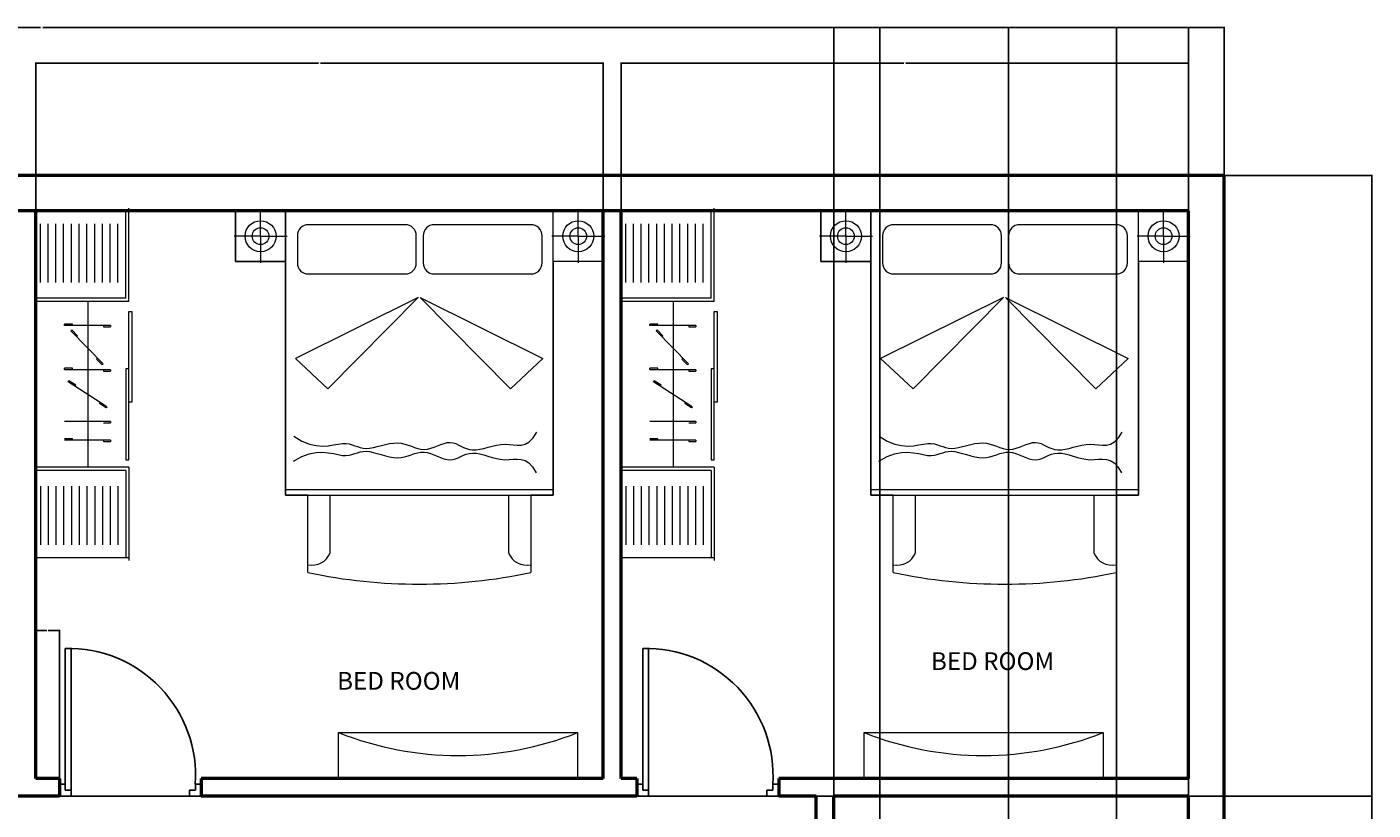
# Model space of a CAD drawing. Units: inches. Extents: x 1865 to 2541, y 1997 to 2759.
# Tile 11 of 11: x 2200 to 2541, y 2560 to 2759. Entities that reach past the tile are written whole.
import ezdxf

# ---------------------------------------------------------------- set-up
doc = ezdxf.new("R2010")
doc.units = ezdxf.units.IN
for name, color, linetype, lineweight in [('A-ANNO-DIMS', 2, 'Continuous', 18), ('A-AREA-IDEN', 4, 'Continuous', 18), ('A-WALL', 7, 'Continuous', 50), ('BED', 42, 'Continuous', 13), ('CUPBOARD', 61, 'Continuous', 18), ('DOOR', 1, 'Continuous', 25), ('TV', 3, 'Continuous', 18)]:
    doc.layers.add(name, color=color, linetype=linetype, lineweight=lineweight)
doc.styles.get("Standard").update_dxf_attribs({"font": 'arial.ttf'})
doc.dimstyles.get("Standard").update_dxf_attribs({"dimtxt": 0.18, "dimasz": 0.18, "dimexe": 0.18, "dimexo": 0.0625, "dimgap": 0.09, "dimtad": 0, "dimtih": 1, "dimtoh": 1, "dimdec": 4, "dimzin": 0, "dimdsep": 46, "dimtxsty": 'Standard', "dimcen": 0.09, "dimadec": 0, "dimazin": 0, "dimtfac": 1, "dimtdec": 4, "dimtofl": 0, "dimtmove": 0, "dimatfit": 3, "dimfxl": 1, "dimtolj": 1, "dimtzin": 0, "dimarcsym": 0})

# ---------------------------------------------------------------- blocks, each defined once
blk = doc.blocks.new('A$C34930FF8')
for p, q in [((600, 1669.3), (600, 2269.3)), ((30, 1790.9), (30, 2169.3)), ((80, 1790.9), (80, 2169.3)), ((130, 1790.9), (130, 2169.3)), ((180, 1790.9), (180, 2169.3)), ((230, 1790.9), (230, 2169.3)), ((280, 1790.9), (280, 2169.3)), ((330, 1790.9), (330, 2169.3)), ((380, 1790.9), (380, 2169.3)), ((430, 1790.9), (430, 2169.3)), ((480, 1790.9), (480, 2169.3)), ((530, 1790.9), (530, 2169.3)), ((580, 1690.9), (580, 2252.4)), ((580, 1690.9), (0, 1690.9)), ((600, 1669.3), (0, 1669.3)), ((335.4, 1666.1), (335.4, 603.1)), ((600, 1603.3), (620, 1603.3)), ((600, 1018.7), (600, 1603.3)), ((620, 1603.3), (620, 1018.7)), ((237.7, 1521.5), (185.4, 1521.5)), ((482.5, 1513), (185.4, 1513)), ((434.8, 1266.1), (227.4, 1478.9)), ((269.7, 1447.7), (233.2, 1485.2)), ((436.7, 1504.4), (482.5, 1504.4)), ((237.7, 1237.7), (185.4, 1237.7)), ((482.5, 1228.2), (185.4, 1228.2)), ((428.7, 1260.1), (392.1, 1297.6)), ((436.7, 1219.7), (482.5, 1219.7)), ((600, 1233.4), (580, 1233.4)), ((580, 1233.4), (580, 648.7)), ((600, 648.7), (600, 1233.4)), ((459.3, 989.3), (209.5, 1150.1)), ((258.1, 1129), (214.1, 1157.3)), ((454.7, 982.1), (410.6, 1010.5)), ((620, 1018.7), (600, 1018.7)), ((482.5, 894.9), (185.4, 894.9)), ((436.7, 886.3), (482.5, 886.3)), ((237.7, 783.9), (185.4, 783.9)), ((482.5, 775.3), (185.4, 775.3)), ((436.7, 766.8), (482.5, 766.8)), ((580, 648.7), (600, 648.7)), ((600, 600), (0, 600)), ((580, 578.3), (0, 578.3)), ((580, 578.3), (580, 16.8)), ((600, 600), (600, 0)), ((30, 478.3), (30, 100)), ((80, 478.3), (80, 100)), ((130, 478.3), (130, 100)), ((180, 478.3), (180, 100)), ((230, 478.3), (230, 100)), ((280, 478.3), (280, 100)), ((330, 478.3), (330, 100)), ((380, 478.3), (380, 100)), ((430, 478.3), (430, 100)), ((480, 478.3), (480, 100)), ((530, 478.3), (530, 100))]:
    blk.add_line(p, q)
at = {"ltscale": 0.05}
for p, q in [((0, 2252.4), (0, 16.8)), ((600, 2252.4), (0, 2252.4)), ((185.4, 1513), (185.4, 1521.5)), ((227.1, 1479.2), (233.2, 1485.2)), ((237.7, 1513), (237.7, 1521.5)), ((436.7, 1513), (436.7, 1504.4)), ((482.5, 1513), (482.5, 1504.4)), ((263.6, 1441.7), (269.7, 1447.7)), ((398.2, 1303.6), (392.1, 1297.6)), ((185.4, 1229.1), (185.4, 1237.7)), ((237.7, 1229.1), (237.7, 1237.7)), ((434.8, 1266.1), (428.7, 1260.1)), ((436.7, 1228.2), (436.7, 1219.7)), ((482.5, 1228.2), (482.5, 1219.7)), ((209.5, 1150.1), (214.1, 1157.3)), ((253.5, 1121.8), (258.1, 1129)), ((415.3, 1017.6), (410.6, 1010.5)), ((459.3, 989.3), (454.7, 982.1)), ((482.5, 894.9), (482.5, 886.3)), ((237.7, 775.3), (237.7, 783.9)), ((436.7, 775.3), (436.7, 766.8)), ((482.5, 775.3), (482.5, 766.8)), ((600, 16.8), (0, 16.8))]:
    blk.add_line(p, q, dxfattribs=at)
blk = doc.blocks.new('A$C4F543DC7')
for p, q in [((0.013, 3.35, -0.169), (3.313, 3.35, -0.169)), ((0.463, 3.35, -0.169), (0.013, 3.35, -0.169)), ((0.013, 2.896, -0.169), (0.013, 3.35, -0.169)), ((0.013, 3.35, -0.169), (0.013, 2.896, -0.169)), ((0.238, 3.123, -0.439), (0.238, 3.361, -0.439)), ((0.463, 3.35, -0.169), (0.463, 0.8, -0.169)), ((2.863, 3.35, -0.169), (0.463, 3.35, -0.169)), ((0.463, 2.896, -0.169), (0.463, 3.35, -0.169)), ((2.863, 0.8, -0.169), (2.863, 3.35, -0.169)), ((2.863, 3.35, -0.169), (3.313, 3.35, -0.169)), ((2.863, 2.896, -0.169), (2.863, 3.35, -0.169)), ((3.089, 3.123, -0.439), (3.089, 3.361, -0.439)), ((3.313, 3.35, -0.169), (3.313, 2.896, -0.169)), ((3.313, 3.35, -0.169), (3.313, 2.896, -0.169)), ((1.535, 3.226, -0.169), (0.668, 3.226, -0.169)), ((2.664, 3.226, -0.169), (1.797, 3.226, -0.169)), ((0.238, 3.123, -0.439), (0, 3.123, -0.439)), ((0.238, 3.123, -0.439), (0.476, 3.123, -0.439)), ((0.238, 3.123, -0.439), (0.238, 2.885, -0.439)), ((0.568, 3.126, -0.169), (0.568, 2.884, -0.169)), ((1.635, 2.884, -0.169), (1.635, 3.126, -0.169)), ((1.697, 3.126, -0.169), (1.697, 2.884, -0.169)), ((2.764, 2.884, -0.169), (2.764, 3.126, -0.169)), ((3.089, 3.123, -0.439), (2.851, 3.123, -0.439)), ((3.089, 3.123, -0.439), (3.089, 2.885, -0.439)), ((3.089, 3.123, -0.439), (3.327, 3.123, -0.439)), ((0.463, 2.896, -0.169), (0.013, 2.896, -0.169)), ((0.013, 2.896, -0.169), (0.463, 2.896, -0.169)), ((0.463, 0.8, -0.169), (0.463, 2.896, -0.169)), ((0.668, 2.784, -0.169), (1.535, 2.784, -0.169)), ((1.797, 2.784, -0.169), (2.664, 2.784, -0.169)), ((2.863, 2.896, -0.169), (2.863, 0.8, -0.169)), ((3.313, 2.896, -0.169), (2.863, 2.896, -0.169)), ((3.313, 2.896, -0.169), (2.863, 2.896, -0.169)), ((1.653, 2.573, -0.169), (0.55, 2.025, -0.169)), ((0.841, 1.752, -0.169), (1.653, 2.573, -0.169)), ((2.481, 1.752, -0.169), (1.669, 2.573, -0.169)), ((1.669, 2.573, -0.169), (2.772, 2.025, -0.169)), ((0.55, 2.025, -0.169), (0.841, 1.752, -0.169)), ((2.772, 2.025, -0.169), (2.481, 1.752, -0.169)), ((2.683, 1.312, -0.169), (2.718, 1.364, -0.169)), ((0.537, 1.327, -0.169), (0.609, 1.284, -0.169)), ((0.609, 1.284, -0.169), (0.676, 1.257, -0.169)), ((0.676, 1.257, -0.169), (0.737, 1.243, -0.169)), ((0.737, 1.243, -0.169), (0.794, 1.239, -0.169)), ((0.794, 1.239, -0.169), (0.846, 1.242, -0.169)), ((0.846, 1.242, -0.169), (0.893, 1.249, -0.169)), ((0.893, 1.249, -0.169), (0.935, 1.256, -0.169)), ((0.935, 1.256, -0.169), (0.972, 1.261, -0.169)), ((0.972, 1.261, -0.169), (1.004, 1.262, -0.169)), ((1.004, 1.262, -0.169), (1.033, 1.258, -0.169)), ((1.033, 1.258, -0.169), (1.06, 1.251, -0.169)), ((1.06, 1.251, -0.169), (1.084, 1.242, -0.169)), ((1.084, 1.242, -0.169), (1.108, 1.234, -0.169)), ((1.108, 1.234, -0.169), (1.132, 1.226, -0.169)), ((1.132, 1.226, -0.169), (1.158, 1.22, -0.169)), ((1.158, 1.22, -0.169), (1.185, 1.218, -0.169)), ((1.185, 1.218, -0.169), (1.216, 1.22, -0.169)), ((1.216, 1.22, -0.169), (1.25, 1.226, -0.169)), ((1.25, 1.226, -0.169), (1.285, 1.235, -0.169)), ((1.285, 1.235, -0.169), (1.322, 1.244, -0.169)), ((1.322, 1.244, -0.169), (1.359, 1.253, -0.169)), ((1.359, 1.253, -0.169), (1.396, 1.261, -0.169)), ((1.396, 1.261, -0.169), (1.433, 1.266, -0.169)), ((1.433, 1.266, -0.169), (1.468, 1.268, -0.169)), ((1.468, 1.268, -0.169), (1.501, 1.264, -0.169)), ((1.501, 1.264, -0.169), (1.532, 1.257, -0.169)), ((1.532, 1.257, -0.169), (1.562, 1.247, -0.169)), ((1.562, 1.247, -0.169), (1.591, 1.237, -0.169)), ((1.591, 1.237, -0.169), (1.62, 1.226, -0.169)), ((1.62, 1.226, -0.169), (1.648, 1.217, -0.169)), ((1.648, 1.217, -0.169), (1.676, 1.211, -0.169)), ((1.676, 1.211, -0.169), (1.705, 1.209, -0.169)), ((1.705, 1.209, -0.169), (1.735, 1.212, -0.169)), ((1.735, 1.212, -0.169), (1.765, 1.22, -0.169)), ((1.765, 1.22, -0.169), (1.795, 1.23, -0.169)), ((1.795, 1.23, -0.169), (1.826, 1.242, -0.169)), ((1.826, 1.242, -0.169), (1.856, 1.253, -0.169)), ((1.856, 1.253, -0.169), (1.885, 1.263, -0.169)), ((1.885, 1.263, -0.169), (1.913, 1.27, -0.169)), ((1.913, 1.27, -0.169), (1.94, 1.272, -0.169)), ((1.94, 1.272, -0.169), (1.965, 1.269, -0.169)), ((1.965, 1.269, -0.169), (1.989, 1.262, -0.169)), ((1.989, 1.262, -0.169), (2.012, 1.251, -0.169)), ((2.012, 1.251, -0.169), (2.036, 1.239, -0.169)), ((2.036, 1.239, -0.169), (2.06, 1.227, -0.169)), ((2.06, 1.227, -0.169), (2.085, 1.216, -0.169)), ((2.085, 1.216, -0.169), (2.112, 1.208, -0.169)), ((2.172, 1.205, -0.169), (2.206, 1.21, -0.169)), ((2.206, 1.21, -0.169), (2.242, 1.218, -0.169)), ((2.242, 1.218, -0.169), (2.279, 1.228, -0.169)), ((2.279, 1.228, -0.169), (2.317, 1.238, -0.169)), ((2.317, 1.238, -0.169), (2.356, 1.246, -0.169)), ((2.356, 1.246, -0.169), (2.394, 1.253, -0.169)), ((2.394, 1.253, -0.169), (2.433, 1.255, -0.169)), ((2.433, 1.255, -0.169), (2.47, 1.253, -0.169)), ((2.47, 1.253, -0.169), (2.506, 1.249, -0.169)), ((2.506, 1.249, -0.169), (2.542, 1.246, -0.169)), ((2.542, 1.246, -0.169), (2.578, 1.248, -0.169)), ((2.578, 1.248, -0.169), (2.613, 1.257, -0.169)), ((2.613, 1.257, -0.169), (2.648, 1.277, -0.169)), ((2.648, 1.277, -0.169), (2.683, 1.312, -0.169)), ((0.533, 1.105, -0.169), (0.607, 1.146, -0.169)), ((0.607, 1.146, -0.169), (0.674, 1.171, -0.169)), ((0.674, 1.171, -0.169), (0.736, 1.183, -0.169)), ((0.736, 1.183, -0.169), (0.793, 1.185, -0.169)), ((0.793, 1.185, -0.169), (0.845, 1.18, -0.169)), ((0.845, 1.18, -0.169), (0.891, 1.172, -0.169)), ((0.891, 1.172, -0.169), (0.933, 1.163, -0.169)), ((0.933, 1.163, -0.169), (0.97, 1.156, -0.169)), ((0.97, 1.156, -0.169), (1.003, 1.155, -0.169)), ((1.003, 1.155, -0.169), (1.032, 1.158, -0.169)), ((1.032, 1.158, -0.169), (1.058, 1.164, -0.169)), ((1.058, 1.164, -0.169), (1.083, 1.172, -0.169)), ((1.083, 1.172, -0.169), (1.107, 1.18, -0.169)), ((1.107, 1.18, -0.169), (1.132, 1.187, -0.169)), ((1.132, 1.187, -0.169), (1.157, 1.192, -0.169)), ((1.157, 1.192, -0.169), (1.185, 1.193, -0.169)), ((1.185, 1.193, -0.169), (1.216, 1.19, -0.169)), ((1.216, 1.19, -0.169), (1.249, 1.183, -0.169)), ((1.249, 1.183, -0.169), (1.284, 1.173, -0.169)), ((1.284, 1.173, -0.169), (1.321, 1.163, -0.169)), ((1.321, 1.163, -0.169), (1.358, 1.152, -0.169)), ((1.358, 1.152, -0.169), (1.394, 1.143, -0.169)), ((1.394, 1.143, -0.169), (1.431, 1.137, -0.169)), ((1.431, 1.137, -0.169), (1.466, 1.135, -0.169)), ((1.466, 1.135, -0.169), (1.499, 1.137, -0.169)), ((1.499, 1.137, -0.169), (1.531, 1.143, -0.169)), ((1.531, 1.143, -0.169), (1.561, 1.152, -0.169)), ((1.561, 1.152, -0.169), (1.59, 1.162, -0.169)), ((1.59, 1.162, -0.169), (1.619, 1.172, -0.169)), ((1.619, 1.172, -0.169), (1.648, 1.18, -0.169)), ((1.648, 1.18, -0.169), (1.676, 1.185, -0.169)), ((1.676, 1.185, -0.169), (1.705, 1.186, -0.169)), ((1.705, 1.186, -0.169), (1.734, 1.182, -0.169)), ((1.734, 1.182, -0.169), (1.764, 1.173, -0.169)), ((1.764, 1.173, -0.169), (1.794, 1.162, -0.169)), ((1.794, 1.162, -0.169), (1.824, 1.149, -0.169)), ((1.824, 1.149, -0.169), (1.854, 1.137, -0.169)), ((1.854, 1.137, -0.169), (1.883, 1.126, -0.169)), ((1.883, 1.126, -0.169), (1.911, 1.119, -0.169)), ((1.911, 1.119, -0.169), (1.937, 1.115, -0.169)), ((1.937, 1.115, -0.169), (1.963, 1.118, -0.169)), ((1.963, 1.118, -0.169), (1.987, 1.124, -0.169)), ((1.987, 1.124, -0.169), (2.011, 1.134, -0.169)), ((2.011, 1.134, -0.169), (2.034, 1.145, -0.169)), ((2.034, 1.145, -0.169), (2.059, 1.157, -0.169)), ((2.059, 1.157, -0.169), (2.084, 1.167, -0.169)), ((2.084, 1.167, -0.169), (2.111, 1.174, -0.169)), ((2.111, 1.174, -0.169), (2.14, 1.177, -0.169)), ((2.112, 1.208, -0.169), (2.141, 1.204, -0.169)), ((2.14, 1.177, -0.169), (2.172, 1.175, -0.169)), ((2.141, 1.204, -0.169), (2.172, 1.205, -0.169)), ((2.172, 1.175, -0.169), (2.206, 1.169, -0.169)), ((2.206, 1.169, -0.169), (2.241, 1.16, -0.169)), ((2.241, 1.16, -0.169), (2.278, 1.149, -0.169)), ((2.278, 1.149, -0.169), (2.316, 1.138, -0.169)), ((2.316, 1.138, -0.169), (2.354, 1.128, -0.169)), ((2.354, 1.128, -0.169), (2.392, 1.121, -0.169)), ((2.392, 1.121, -0.169), (2.43, 1.117, -0.169)), ((2.43, 1.117, -0.169), (2.468, 1.118, -0.169)), ((2.468, 1.118, -0.169), (2.504, 1.121, -0.169)), ((2.504, 1.121, -0.169), (2.54, 1.123, -0.169)), ((2.54, 1.123, -0.169), (2.576, 1.12, -0.169)), ((2.576, 1.12, -0.169), (2.611, 1.109, -0.169)), ((2.611, 1.109, -0.169), (2.645, 1.088, -0.169)), ((2.645, 1.088, -0.169), (2.679, 1.052, -0.169)), ((2.679, 1.052, -0.169), (2.712, 0.999, -0.169)), ((0.463, 0.85, -0.169), (2.863, 0.85, -0.169)), ((0.463, 0.8, -0.169), (2.863, 0.8, -0.169)), ((0.663, 0.8, -0.169), (0.463, 0.8, -0.169)), ((0.663, 0.8, -0.169), (2.663, 0.8, -0.169)), ((0.663, 0.104, -0.169), (0.663, 0.8, -0.169)), ((0.663, 0.104, -0.169), (0.663, 0.8, -0.169)), ((0.863, 0.281, -0.169), (0.863, 0.8, -0.169)), ((2.463, 0.8, -0.169), (2.463, 0.281, -0.169)), ((2.863, 0.8, -0.169), (2.663, 0.8, -0.169)), ((2.663, 0.8, -0.169), (2.663, 0.104, -0.169)), ((2.663, 0.8, -0.169), (2.663, 0.104, -0.169))]:
    blk.add_line(p, q)
for centre, radius in [((0.238, 3.123, -0.439), 0.139), ((3.089, 3.123, -0.439), 0.139), ((0.238, 3.123, -0.439), 0.075), ((3.089, 3.123, -0.439), 0.075)]:
    blk.add_circle(centre, radius)
for centre, radius, start, end in [((0.668, 3.126, -0.169), 0.1, 90, 180), ((1.535, 3.126, -0.169), 0.1, 0, 90), ((1.797, 3.126, -0.169), 0.1, 90, 180), ((2.664, 3.126, -0.169), 0.1, 0, 90), ((0.668, 2.884, -0.169), 0.1, 180, 270), ((1.535, 2.884, -0.169), 0.1, 270, 0), ((1.797, 2.884, -0.169), 0.1, 180, 270), ((2.664, 2.884, -0.169), 0.1, 270, 0), ((0.699, 0.347, -0.169), 0.177, 258.2616, 338.032), ((2.627, 0.347, -0.169), 0.177, 201.968, 281.7384), ((1.663, 4.86, -0.169), 4.86, 258.1252, 281.8748), ((1.663, 4.86, -0.169), 4.86, 258.1252, 281.8748)]:
    blk.add_arc(centre, radius, start, end)
blk = doc.blocks.new('DOOR-SWING-36IN')
for p, q in [((36.01, 34.5), (0.01, 34.5)), ((34.51, 36), (37.51, 36)), ((34.51, 34.5), (34.51, 36)), ((36.01, 34.5), (34.51, 34.5)), ((36.01, 33), (36.01, 34.5)), ((37.51, 36), (37.51, 33)), ((36.01, 33), (0.01, 33)), ((37.51, 33), (36.01, 33)), ((36.01, 1.5), (34.51, 1.5)), ((34.51, 1.5), (34.51, 0)), ((34.51, 0), (37.51, 0)), ((37.51, 3), (36.01, 3)), ((36.01, 3), (36.01, 1.5)), ((37.51, 0), (37.51, 3))]:
    blk.add_line(p, q)
blk.add_arc((32.32, 33.75), 32.32, 178.6705, 273.8756)
blk = doc.blocks.new('TV-UNIT')
blk.add_lwpolyline([(0, 11.62), (60.65, 11.62), (60.65, 0), (0, 0)], close=True)
blk.add_arc((30.32, -76.26), 82.06, 68.3146, 111.6854)
blk = doc.blocks.new('*D40')
at = {"layer": 'A-ANNO-DIMS', "color": 0, "lineweight": -2, "transparency": 16777216}
for p, q in [((1903.24, 2721.51), (1903.24, 2759.13)), ((1903.42, 2758.95), (2202.95, 2758.95)), ((2503.06, 2758.95), (2203.53, 2758.95)), ((2503.24, 2721.51), (2503.24, 2759.13))]:
    blk.add_line(p, q, dxfattribs=at)
at = {"layer": 'A-ANNO-DIMS', "color": 0, "transparency": 16777216}
for points in [[(1903.42, 2758.98), (1903.42, 2758.92), (1903.24, 2758.95)], [(2503.06, 2758.98), (2503.06, 2758.92), (2503.24, 2758.95)]]:
    blk.add_solid(points, dxfattribs=at)
at = {"layer": 'Defpoints', "color": 0, "transparency": 16777216}
for p in [(2503.24, 2758.95), (1903.24, 2721.45), (2503.24, 2721.45)]:
    blk.add_point(p, dxfattribs=at)
at = {"layer": 'A-ANNO-DIMS', "color": 0, "transparency": 16777216, "insert": (2203.24, 2758.95), "char_height": 0.18, "attachment_point": 5}
blk.add_mtext('\\A1;600', dxfattribs=at)
blk = doc.blocks.new('*D41')
at = {"layer": 'A-ANNO-DIMS', "color": 0, "lineweight": -2, "transparency": 16777216}
for p, q in [((2503.31, 2721.45), (2540.92, 2721.45)), ((2540.74, 2721.27), (2540.74, 2378.49)), ((2540.74, 2035.35), (2540.74, 2378.13)), ((2136.19, 2035.17), (2540.92, 2035.17))]:
    blk.add_line(p, q, dxfattribs=at)
at = {"layer": 'A-ANNO-DIMS', "color": 0, "transparency": 16777216}
for points in [[(2540.71, 2721.27), (2540.77, 2721.27), (2540.74, 2721.45)], [(2540.71, 2035.35), (2540.77, 2035.35), (2540.74, 2035.17)]]:
    blk.add_solid(points, dxfattribs=at)
at = {"layer": 'Defpoints', "color": 0, "transparency": 16777216}
for p in [(2503.24, 2721.45), (2136.13, 2035.17), (2540.74, 2035.17)]:
    blk.add_point(p, dxfattribs=at)
at = {"layer": 'A-ANNO-DIMS', "color": 0, "transparency": 16777216, "insert": (2540.74, 2378.31), "char_height": 0.18, "attachment_point": 5}
blk.add_mtext('\\A1;686.3', dxfattribs=at)
blk = doc.blocks.new('*D45')
at = {"layer": 'A-ANNO-DIMS', "color": 0, "lineweight": -2, "transparency": 16777216}
for p, q in [((2201.74, 2712.51), (2201.74, 2750.13)), ((2201.92, 2749.95), (2273.46, 2749.95)), ((2345.56, 2749.95), (2274.02, 2749.95)), ((2345.74, 2712.51), (2345.74, 2750.13))]:
    blk.add_line(p, q, dxfattribs=at)
at = {"layer": 'A-ANNO-DIMS', "color": 0, "transparency": 16777216}
for points in [[(2201.92, 2749.98), (2201.92, 2749.92), (2201.74, 2749.95)], [(2345.56, 2749.98), (2345.56, 2749.92), (2345.74, 2749.95)]]:
    blk.add_solid(points, dxfattribs=at)
at = {"layer": 'Defpoints', "color": 0, "transparency": 16777216}
for p in [(2345.74, 2749.95), (2201.74, 2712.45), (2345.74, 2712.45)]:
    blk.add_point(p, dxfattribs=at)
at = {"layer": 'A-ANNO-DIMS', "color": 0, "transparency": 16777216, "insert": (2273.74, 2749.95), "char_height": 0.18, "attachment_point": 5}
blk.add_mtext('\\A1;144', dxfattribs=at)
blk = doc.blocks.new('*D46')
at = {"layer": 'A-ANNO-DIMS', "color": 0, "lineweight": -2, "transparency": 16777216}
for p, q in [((2350.24, 2712.51), (2350.24, 2750.13)), ((2350.42, 2749.95), (2421.96, 2749.95)), ((2494.06, 2749.95), (2422.52, 2749.95)), ((2494.24, 2712.51), (2494.24, 2750.13))]:
    blk.add_line(p, q, dxfattribs=at)
at = {"layer": 'A-ANNO-DIMS', "color": 0, "transparency": 16777216}
for points in [[(2350.42, 2749.98), (2350.42, 2749.92), (2350.24, 2749.95)], [(2494.06, 2749.98), (2494.06, 2749.92), (2494.24, 2749.95)]]:
    blk.add_solid(points, dxfattribs=at)
at = {"layer": 'Defpoints', "color": 0, "transparency": 16777216}
for p in [(2494.24, 2749.95), (2350.24, 2712.45), (2494.24, 2712.45)]:
    blk.add_point(p, dxfattribs=at)
at = {"layer": 'A-ANNO-DIMS', "color": 0, "transparency": 16777216, "insert": (2422.24, 2749.95), "char_height": 0.18, "attachment_point": 5}
blk.add_mtext('\\A1;144', dxfattribs=at)
blk = doc.blocks.new('*D61')
at = {"layer": 'A-ANNO-DIMS', "color": 0, "lineweight": -2, "transparency": 16777216}
for p, q in [((2404.24, 2564.01), (2404.24, 2759.13)), ((2404.42, 2758.95), (2449.02, 2758.95)), ((2494.06, 2758.95), (2449.46, 2758.95)), ((2494.24, 2564.01), (2494.24, 2759.13))]:
    blk.add_line(p, q, dxfattribs=at)
at = {"layer": 'A-ANNO-DIMS', "color": 0, "transparency": 16777216}
for points in [[(2404.42, 2758.98), (2404.42, 2758.92), (2404.24, 2758.95)], [(2494.06, 2758.98), (2494.06, 2758.92), (2494.24, 2758.95)]]:
    blk.add_solid(points, dxfattribs=at)
at = {"layer": 'Defpoints', "color": 0, "transparency": 16777216}
for p in [(2494.24, 2758.95), (2404.24, 2563.95), (2494.24, 2563.95)]:
    blk.add_point(p, dxfattribs=at)
at = {"layer": 'A-ANNO-DIMS', "color": 0, "transparency": 16777216, "insert": (2449.24, 2758.95), "char_height": 0.18, "attachment_point": 5}
blk.add_mtext('\\A1;90', dxfattribs=at)
blk = doc.blocks.new('*D62')
at = {"layer": 'A-ANNO-DIMS', "color": 0, "lineweight": -2, "transparency": 16777216}
for p, q in [((2494.31, 2563.95), (2540.92, 2563.95)), ((2540.74, 2563.77), (2540.74, 2485.63)), ((2540.74, 2407.13), (2540.74, 2485.27)), ((2494.31, 2406.95), (2540.92, 2406.95))]:
    blk.add_line(p, q, dxfattribs=at)
at = {"layer": 'A-ANNO-DIMS', "color": 0, "transparency": 16777216}
for points in [[(2540.71, 2563.77), (2540.77, 2563.77), (2540.74, 2563.95)], [(2540.71, 2407.13), (2540.77, 2407.13), (2540.74, 2406.95)]]:
    blk.add_solid(points, dxfattribs=at)
at = {"layer": 'Defpoints', "color": 0, "transparency": 16777216}
for p in [(2494.24, 2563.95), (2540.74, 2563.95), (2494.24, 2406.95)]:
    blk.add_point(p, dxfattribs=at)
at = {"layer": 'A-ANNO-DIMS', "color": 0, "transparency": 16777216, "insert": (2540.74, 2485.45), "char_height": 0.18, "attachment_point": 5}
blk.add_mtext('\\A1;157', dxfattribs=at)
blk = doc.blocks.new('*D63')
at = {"layer": 'A-ANNO-DIMS', "color": 0, "lineweight": -2, "transparency": 16777216}
for p, q in [((2404.18, 2563.95), (1865.56, 2563.95)), ((1865.74, 2563.77), (1865.74, 2538.51)), ((1865.74, 2512.9), (1865.74, 2538.15)), ((2404.18, 2512.72), (1865.56, 2512.72))]:
    blk.add_line(p, q, dxfattribs=at)
at = {"layer": 'A-ANNO-DIMS', "color": 0, "transparency": 16777216}
for points in [[(1865.71, 2563.77), (1865.77, 2563.77), (1865.74, 2563.95)], [(1865.71, 2512.9), (1865.77, 2512.9), (1865.74, 2512.72)]]:
    blk.add_solid(points, dxfattribs=at)
at = {"layer": 'Defpoints', "color": 0, "transparency": 16777216}
for p in [(2404.24, 2563.95), (1865.74, 2512.72), (2404.24, 2512.72)]:
    blk.add_point(p, dxfattribs=at)
at = {"layer": 'A-ANNO-DIMS', "color": 0, "transparency": 16777216, "insert": (1865.74, 2538.33), "char_height": 0.18, "attachment_point": 5}
blk.add_mtext('\\A1;51.23', dxfattribs=at)
blk = doc.blocks.new('*D65')
at = {"layer": 'A-ANNO-DIMS', "color": 0, "lineweight": -2, "transparency": 16777216}
for p, q in [((2475.95, 2510.05), (2475.95, 2759.13)), ((2476.13, 2758.95), (2484.71, 2758.95)), ((2494.06, 2758.95), (2485.48, 2758.95)), ((2494.24, 2510.05), (2494.24, 2759.13))]:
    blk.add_line(p, q, dxfattribs=at)
at = {"layer": 'A-ANNO-DIMS', "color": 0, "transparency": 16777216}
for points in [[(2476.13, 2758.98), (2476.13, 2758.92), (2475.95, 2758.95)], [(2494.06, 2758.98), (2494.06, 2758.92), (2494.24, 2758.95)]]:
    blk.add_solid(points, dxfattribs=at)
at = {"layer": 'Defpoints', "color": 0, "transparency": 16777216}
for p in [(2494.24, 2758.95), (2475.95, 2509.99), (2494.24, 2509.99)]:
    blk.add_point(p, dxfattribs=at)
at = {"layer": 'A-ANNO-DIMS', "color": 0, "transparency": 16777216, "insert": (2485.1, 2758.95), "char_height": 0.18, "attachment_point": 5}
blk.add_mtext('\\A1;18.29', dxfattribs=at)
blk = doc.blocks.new('*D77')
at = {"layer": 'A-ANNO-DIMS', "color": 0, "lineweight": -2, "transparency": 16777216}
for p, q in [((2415.89, 2419.2), (2415.89, 2759.13)), ((2416.07, 2758.95), (2431.92, 2758.95)), ((2448.41, 2758.95), (2432.57, 2758.95)), ((2448.59, 2419.2), (2448.59, 2759.13))]:
    blk.add_line(p, q, dxfattribs=at)
at = {"layer": 'A-ANNO-DIMS', "color": 0, "transparency": 16777216}
for points in [[(2416.07, 2758.98), (2416.07, 2758.92), (2415.89, 2758.95)], [(2448.41, 2758.98), (2448.41, 2758.92), (2448.59, 2758.95)]]:
    blk.add_solid(points, dxfattribs=at)
at = {"layer": 'Defpoints', "color": 0, "transparency": 16777216}
for p in [(2448.59, 2758.95), (2415.89, 2419.14), (2448.59, 2419.14)]:
    blk.add_point(p, dxfattribs=at)
at = {"layer": 'A-ANNO-DIMS', "color": 0, "transparency": 16777216, "insert": (2432.24, 2758.95), "char_height": 0.18, "attachment_point": 5}
blk.add_mtext('\\A1;32.7', dxfattribs=at)
blk = doc.blocks.new('*D80')
at = {"layer": 'A-ANNO-DIMS', "color": 0, "lineweight": -2, "transparency": 16777216}
for p, q in [((2201.74, 2568.51), (2201.74, 2606.13)), ((2201.92, 2605.95), (2204.59, 2605.95)), ((2207.56, 2605.95), (2204.89, 2605.95)), ((2207.74, 2568.51), (2207.74, 2606.13))]:
    blk.add_line(p, q, dxfattribs=at)
at = {"layer": 'A-ANNO-DIMS', "color": 0, "transparency": 16777216}
for points in [[(2201.92, 2605.98), (2201.92, 2605.92), (2201.74, 2605.95)], [(2207.56, 2605.98), (2207.56, 2605.92), (2207.74, 2605.95)]]:
    blk.add_solid(points, dxfattribs=at)
at = {"layer": 'Defpoints', "color": 0, "transparency": 16777216}
for p in [(2207.74, 2605.95), (2201.74, 2568.45), (2207.74, 2568.45)]:
    blk.add_point(p, dxfattribs=at)
at = {"layer": 'A-ANNO-DIMS', "color": 0, "transparency": 16777216, "insert": (2204.74, 2605.95), "char_height": 0.18, "attachment_point": 5}
blk.add_mtext('\\A1;6', dxfattribs=at)

msp = doc.modelspace()

# ---------------------------------------------------------------- linework, layer by layer
at = {"layer": 'A-WALL'}
for p, q in [((2503.243, 2721.4494), (1903.243, 2721.4494)), ((2503.243, 2061.4494), (2503.243, 2721.4494)), ((2494.243, 2712.4494), (2161.2838, 2712.4494)), ((2201.743, 2568.4494), (2201.743, 2712.4494)), ((2345.743, 2568.4494), (2345.743, 2712.4494)), ((2345.743, 2568.4494), (2345.743, 2712.4494)), ((2350.243, 2568.4494), (2350.243, 2712.4494)), ((2350.243, 2568.4494), (2350.243, 2712.4494)), ((2494.243, 2568.4494), (2494.243, 2712.4494)), ((2207.743, 2568.4494), (2201.743, 2568.4494)), ((2207.743, 2568.4494), (2207.743, 2563.9494)), ((2345.743, 2568.4494), (2243.743, 2568.4494)), ((2243.743, 2568.4494), (2243.743, 2563.9494)), ((2354.243, 2568.4494), (2350.243, 2568.4494)), ((2354.243, 2568.4494), (2354.243, 2563.9494)), ((2494.243, 2568.4494), (2390.243, 2568.4494)), ((2390.243, 2568.4494), (2390.243, 2563.9494)), ((2207.743, 2563.9494), (2197.243, 2563.9494)), ((2354.243, 2563.9494), (2243.743, 2563.9494)), ((2399.743, 2563.9494), (2390.243, 2563.9494)), ((2399.743, 2512.7166), (2399.743, 2563.9494)), ((2494.243, 2563.9494), (2404.243, 2563.9494)), ((2404.243, 2512.7166), (2404.243, 2563.9494)), ((2494.243, 2406.9494), (2494.243, 2563.9494))]:
    msp.add_line(p, q, dxfattribs=at)

# ---------------------------------------------------------------- block references
at = {"layer": 'BED', "xscale": 28.27205529407425, "yscale": 28.27205529407425, "zscale": 28.27205529407425}
for p in [(2252.0653, 2617.738, 4.7709), (2400.5653, 2617.738, 4.7709)]:
    msp.add_blockref('A$C4F543DC7', p, dxfattribs=at)
at = {"layer": 'CUPBOARD', "xscale": 0.0393700787401575, "yscale": 0.0393700787401575, "zscale": 0.0393700787401575}
for p in [(2201.743, 2623.7716), (2350.243, 2623.7716)]:
    msp.add_blockref('A$C34930FF8', p, dxfattribs=at)
at = {"layer": 'DOOR', "extrusion": (0, 0, -1), "zscale": -1}
for p, rotation in [((-2243.7434, 2601.4584), 269.9999999999814), ((-2390.2434, 2601.4584), 269.9999999999787)]:
    msp.add_blockref('DOOR-SWING-36IN', p, dxfattribs=dict(at, rotation=rotation))
at = {"layer": 'TV', "rotation": 180}
for p in [(2339.2234, 2580.0649), (2472.5659, 2580.0649)]:
    msp.add_blockref('TV-UNIT', p, dxfattribs=at)

# ---------------------------------------------------------------- texts
at = {"layer": 'A-AREA-IDEN', "char_height": 4.5, "attachment_point": 1}
for insert in [(2428.8768, 2600.4538), (2278.2224, 2595.4546)]:
    msp.add_mtext_dynamic_manual_height_columns('BED ROOM', width=66.075761, gutter_width=12.5, heights=[0], dxfattribs=dict(at, insert=insert))

# ---------------------------------------------------------------- dimensions: what is measured, and where the dimension line sits
at = {"layer": 'A-ANNO-DIMS'}
for base, p1, p2, override, picture, middle in [((2503.243, 2758.9494), (1903.243, 2721.4494), (2503.243, 2721.4494), {"dimdec": 0, "dimlfac": 1, "dimrnd": 0, "dimzin": 0, "dimdsep": 46, "dimlunit": 2}, '*D40', (2203.243, 2758.9494)), ((2494.243, 2758.9494), (2404.243, 2563.9494), (2494.243, 2563.9494), {"dimdec": 0, "dimlfac": 1, "dimrnd": 0, "dimzin": 0, "dimdsep": 46, "dimlunit": 2}, '*D61', (2449.243, 2758.9494)), ((2448.5933, 2758.9494), (2415.893, 2419.142), (2448.5933, 2419.142), {"dimdec": 1, "dimlfac": 1, "dimrnd": 0, "dimzin": 0, "dimdsep": 46, "dimlunit": 2}, '*D77', (2432.2431, 2758.9494)), ((2494.243, 2758.9494), (2475.9518, 2509.9875), (2494.243, 2509.9875), {"dimdec": 2, "dimlfac": 1, "dimrnd": 0, "dimzin": 0, "dimdsep": 46, "dimlunit": 2}, '*D65', (2485.0974, 2758.9494)), ((2345.743, 2749.9494), (2201.743, 2712.4494), (2345.743, 2712.4494), {"dimdec": 0, "dimlfac": 1, "dimrnd": 0, "dimzin": 0, "dimdsep": 46, "dimlunit": 2}, '*D45', (2273.743, 2749.9494)), ((2207.743, 2605.9494), (2201.743, 2568.4494), (2207.743, 2568.4494), {"dimdec": 0, "dimlfac": 1, "dimrnd": 0, "dimzin": 0, "dimdsep": 46, "dimlunit": 2}, '*D80', (2204.743, 2605.9494))]:
    dim = msp.add_linear_dim(base=base, p1=p1, p2=p2, dimstyle='Standard', override=override, dxfattribs=at)
    dim.commit()
    dim.dimension.update_dxf_attribs({"geometry": picture, "text_midpoint": middle})
for base, p1, p2, angle, override, picture, middle in [((2494.243, 2749.9494), (2350.243, 2712.4494), (2494.243, 2712.4494), 0, {"dimdec": 0, "dimlfac": 1, "dimrnd": 0, "dimzin": 0, "dimdsep": 46, "dimlunit": 2}, '*D46', (2422.243, 2749.9494)), ((2540.743, 2035.1708), (2503.243, 2721.4494), (2136.13, 2035.1708), 90, {"dimdec": 1, "dimlfac": 1, "dimrnd": 0, "dimzin": 0, "dimdsep": 46, "dimlunit": 2}, '*D41', (2540.743, 2378.3101)), ((1865.743, 2512.7166), (2404.243, 2563.9494), (2404.243, 2512.7166), 90, {"dimdec": 2, "dimlfac": 1, "dimrnd": 0, "dimzin": 0, "dimdsep": 46, "dimlunit": 2}, '*D63', (1865.743, 2538.333)), ((2540.743, 2563.9494), (2494.243, 2406.9494), (2494.243, 2563.9494), 90, {"dimdec": 0, "dimlfac": 1, "dimrnd": 0, "dimzin": 0, "dimdsep": 46, "dimlunit": 2}, '*D62', (2540.743, 2485.4494))]:
    dim = msp.add_linear_dim(base=base, p1=p1, p2=p2, angle=angle, dimstyle='Standard', override=override, dxfattribs=at)
    dim.commit()
    dim.dimension.update_dxf_attribs({"geometry": picture, "text_midpoint": middle})

doc.saveas('drawing.dxf')
